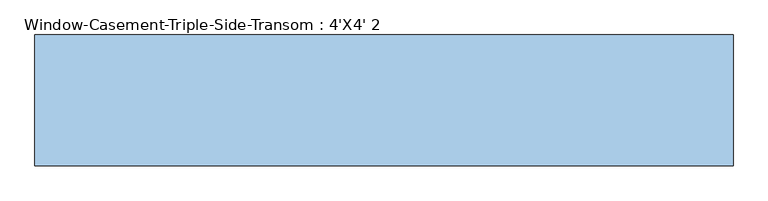
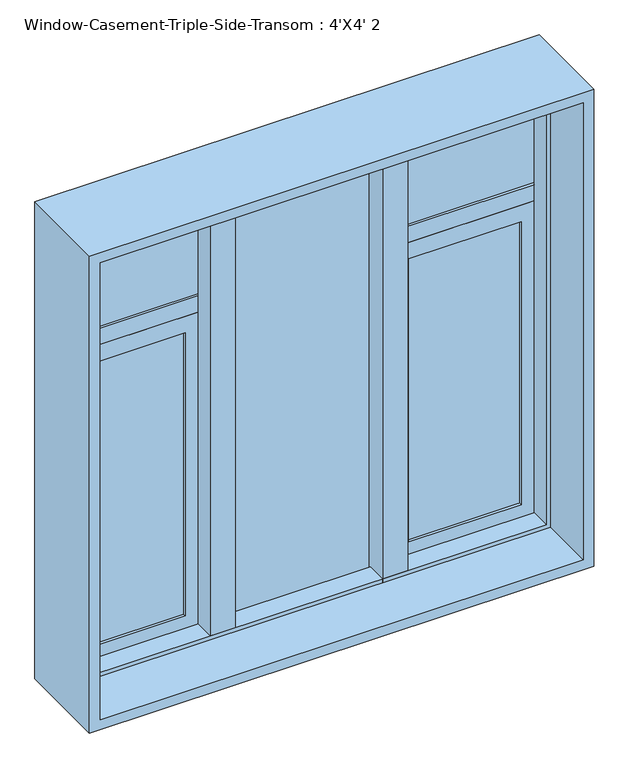
"""IFC4 building model written with IfcOpenShell, lengths in millimetres: window geometry, Window-Casement-Triple-Side-Transom : 4'X4' 2."""

from ifc_helpers import new_model, si_unit, frame, origin, place, context, project, spatial, polyline, outline, extrude, faceted_brep, source, transform, mapped, element, save


def window_casement_triple_side_transom_4_x4_2_fd24aed3(model_context):
    return source(origin(), model_context, "Body", "SolidModel", [
        faceted_brep([(-584.2, 73.025, 2108.2), (-584.2, 114.3, 2108.2), (584.2, 114.3, 2108.2), (584.2, 73.025, 2108.2), (-574.0796875, 22.225, 2098.0796875), (-574.0796875, 73.025, 2098.0796875), (574.0796875, 73.025, 2098.0796875), (574.0796875, 22.225, 2098.0796875), (-584.2, -114.3, 2108.2), (-584.2, 22.225, 2108.2), (584.2, 22.225, 2108.2), (584.2, -114.3, 2108.2), (-609.6, 114.3, 2133.6), (-609.6, -114.3, 2133.6), (609.6, -114.3, 2133.6), (609.6, 114.3, 2133.6), (584.2, 114.3, 939.8), (584.2, 73.025, 939.8), (574.0796875, 73.025, 949.9203125), (574.0796875, 22.225, 949.9203125), (584.2, 22.225, 939.8), (584.2, -114.3, 939.8), (609.6, -114.3, 914.4), (609.6, 114.3, 914.4), (-584.2, 114.3, 939.8), (-584.2, 73.025, 939.8), (-574.0796875, 73.025, 949.9203125), (-574.0796875, 22.225, 949.9203125), (-584.2, 22.225, 939.8), (-584.2, -114.3, 939.8), (-609.6, -114.3, 914.4), (-609.6, 114.3, 914.4)], [[[0, 1, 2, 3]], [[4, 5, 6, 7]], [[8, 9, 10, 11]], [[12, 13, 14, 15]], [[3, 2, 16, 17]], [[7, 6, 18, 19]], [[11, 10, 20, 21]], [[15, 14, 22, 23]], [[17, 16, 24, 25]], [[19, 18, 26, 27]], [[21, 20, 28, 29]], [[23, 22, 30, 31]], [[25, 24, 1, 0]], [[3, 17, 25, 0], [5, 26, 18, 6]], [[27, 26, 5, 4]], [[9, 28, 20, 10], [7, 19, 27, 4]], [[29, 28, 9, 8]], [[13, 30, 22, 14], [11, 21, 29, 8]], [[31, 30, 13, 12]], [[15, 23, 31, 12], [1, 24, 16, 2]]]),
        extrude(outline(polyline([(-177.8, 111.125), (-177.8, 22.225), (-238.7203125, 22.225), (-238.7203125, 73.025), (-228.6, 73.025), (-228.6, 111.125), (-177.8, 111.125)])), frame((0.0, 0.0, 939.8), z_axis=(0.0, 0.0, 1.0), x_axis=(1.0, 0.0, 0.0)), (0.0, 0.0, 1.0), 1168.4),
        extrude(outline(polyline([(228.6, 111.125), (228.6, 73.025), (238.7203125, 73.025), (238.7203125, 22.225), (177.8, 22.225), (177.8, 111.125), (228.6, 111.125)])), frame((0.0, 0.0, 939.8), z_axis=(0.0, 0.0, 1.0), x_axis=(1.0, 0.0, 0.0)), (0.0, 0.0, 1.0), 1168.4),
        extrude(outline(polyline([(1746.9048438, 228.6), (939.8, 228.6), (939.8, 584.2), (1746.9048438, 584.2), (1746.9048438, 228.6)]), holes=[polyline([(1705.0345313, 542.3296875), (981.6703125, 542.3296875), (981.6703125, 270.4703125), (1705.0345313, 270.4703125), (1705.0345313, 542.3296875)])]), frame((0.0, 73.025, 0.0), z_axis=(0.0, 1.0, 0.0), x_axis=(0.0, 0.0, 1.0)), (0.0, 0.0, 1.0), 31.75),
        extrude(outline(polyline([(1746.9048438, -584.2), (939.8, -584.2), (939.8, -228.6), (1746.9048438, -228.6), (1746.9048438, -584.2)]), holes=[polyline([(1705.0345313, -270.4703125), (981.6703125, -270.4703125), (981.6703125, -542.3296875), (1705.0345313, -542.3296875), (1705.0345313, -270.4703125)])]), frame((0.0, 73.025, 0.0), z_axis=(0.0, 1.0, 0.0), x_axis=(0.0, 0.0, 1.0)), (0.0, 0.0, 1.0), 31.75),
        extrude(outline(polyline([(-270.4703125, 98.425), (-270.4703125, 92.075), (-542.3296875, 92.075), (-542.3296875, 98.425), (-270.4703125, 98.425)])), frame((0.0, 0.0, 981.6703125), z_axis=(0.0, 0.0, 1.0), x_axis=(1.0, 0.0, 0.0)), (0.0, 0.0, 1.0), 723.3642188),
        extrude(outline(polyline([(-270.4703125, 85.725), (-270.4703125, 79.375), (-542.3296875, 79.375), (-542.3296875, 85.725), (-270.4703125, 85.725)])), frame((0.0, 0.0, 981.6703125), z_axis=(0.0, 0.0, 1.0), x_axis=(1.0, 0.0, 0.0)), (0.0, 0.0, 1.0), 723.3642188),
        extrude(outline(polyline([(542.3296875, 98.425), (542.3296875, 92.075), (270.4703125, 92.075), (270.4703125, 98.425), (542.3296875, 98.425)])), frame((0.0, 0.0, 981.6703125), z_axis=(0.0, 0.0, 1.0), x_axis=(1.0, 0.0, 0.0)), (0.0, 0.0, 1.0), 723.3642188),
        extrude(outline(polyline([(542.3296875, 85.725), (542.3296875, 79.375), (270.4703125, 79.375), (270.4703125, 85.725), (542.3296875, 85.725)])), frame((0.0, 0.0, 981.6703125), z_axis=(0.0, 0.0, 1.0), x_axis=(1.0, 0.0, 0.0)), (0.0, 0.0, 1.0), 723.3642188),
        extrude(outline(polyline([(584.2, 104.775), (584.2, 73.025), (228.6, 73.025), (228.6, 104.775), (584.2, 104.775)])), frame((0.0, 0.0, 1746.9048438), z_axis=(0.0, 0.0, 1.0), x_axis=(1.0, 0.0, 0.0)), (0.0, 0.0, 1.0), 41.8703125),
        extrude(outline(polyline([(177.8, 98.425), (177.8, 92.075), (-177.8, 92.075), (-177.8, 98.425), (177.8, 98.425)])), frame((0.0, 0.0, 939.8), z_axis=(0.0, 0.0, 1.0), x_axis=(1.0, 0.0, 0.0)), (0.0, 0.0, 1.0), 1168.4),
        extrude(outline(polyline([(177.8, 85.725), (177.8, 79.375), (-177.8, 79.375), (-177.8, 85.725), (177.8, 85.725)])), frame((0.0, 0.0, 939.8), z_axis=(0.0, 0.0, 1.0), x_axis=(1.0, 0.0, 0.0)), (0.0, 0.0, 1.0), 1168.4),
        extrude(outline(polyline([(-228.6, 104.775), (-228.6, 73.025), (-584.2, 73.025), (-584.2, 104.775), (-228.6, 104.775)])), frame((0.0, 0.0, 1746.9048438), z_axis=(0.0, 0.0, 1.0), x_axis=(1.0, 0.0, 0.0)), (0.0, 0.0, 1.0), 41.8703125),
        extrude(outline(polyline([(-228.6, 98.425), (-228.6, 92.075), (-584.2, 92.075), (-584.2, 98.425), (-228.6, 98.425)])), frame((0.0, 0.0, 1788.7751562), z_axis=(0.0, 0.0, 1.0), x_axis=(1.0, 0.0, 0.0)), (0.0, 0.0, 1.0), 319.4248438),
        extrude(outline(polyline([(-228.6, 85.725), (-228.6, 79.375), (-584.2, 79.375), (-584.2, 85.725), (-228.6, 85.725)])), frame((0.0, 0.0, 1788.7751562), z_axis=(0.0, 0.0, 1.0), x_axis=(1.0, 0.0, 0.0)), (0.0, 0.0, 1.0), 319.4248438),
        extrude(outline(polyline([(584.2, 98.425), (584.2, 92.075), (228.6, 92.075), (228.6, 98.425), (584.2, 98.425)])), frame((0.0, 0.0, 1788.7751562), z_axis=(0.0, 0.0, 1.0), x_axis=(1.0, 0.0, 0.0)), (0.0, 0.0, 1.0), 319.4248438),
        extrude(outline(polyline([(584.2, 85.725), (584.2, 79.375), (228.6, 79.375), (228.6, 85.725), (584.2, 85.725)])), frame((0.0, 0.0, 1788.7751562), z_axis=(0.0, 0.0, 1.0), x_axis=(1.0, 0.0, 0.0)), (0.0, 0.0, 1.0), 319.4248438),
    ])


if __name__ == "__main__":
    model = new_model("IFC4")
    model_context = context("Model", 3, world=origin())
    ifc_project = project(units=[si_unit("LENGTHUNIT", "METRE", prefix="MILLI")], contexts=[model_context])
    site = spatial("IfcSite", under=ifc_project)
    building = spatial("IfcBuilding", under=site)
    placement = place(None, origin())
    window_casement_triple_side_transom_4_x4_2_shape = window_casement_triple_side_transom_4_x4_2_fd24aed3(model_context)
    element("IfcWindow", 1, ObjectType="Window-Casement-Triple-Side-Transom : 4'X4' 2", at=placement, inside=building, context=model_context, shape_type="MappedRepresentation", body=[
        mapped(window_casement_triple_side_transom_4_x4_2_shape, transform((0.0, 0.0, 0.0), x_axis=(1.0, 0.0, 0.0), y_axis=(0.0, 1.0, 0.0), z_axis=(0.0, 0.0, 1.0))),
    ])
    save(model, "model.ifc")

# Revit data of these elements
# Type "Window-Casement-Triple-Side-Transom : 4'X4' 2"
#   Type Mark = "26"
#   Fire Rating = "0.5h"
#   Assembly Code = "B2020100"
#   Analytic Construction = "Double glazing - domestic"
#   Window Width = 1' - 4"
#   Window Inset [instance default] = 0' - 0 5/8"
#   Wall Thickness [instance default] = 0' - 6"
#   Visual Light Transmittance = 0.81
#   Transom Height Ratio = 0.3
#   Thermal Resistance (R) = 1.8146 (h·ft²·°F)/BTU
#   Solar Heat Gain Coefficient = 0.76
#   Rough Width = 4' - 0 1/2"
#   Rough Height = 4' - 0 1/2"
#   Open Window Height = 2' - 9.6"
#   Heat Transfer Coefficient (U) = 0.5511 BTU/(h·ft²·°F)
#   Height = 4' - 0"
#   Transom Height = 1' - 2.4"
#   Frame Gap 3 [instance default] = 0' - 1 83/128"
#   Frame Gap 2 [instance default] = 0' - 0 5/8"
#   Frame Gap 1 = 0' - 1 51/128"
#   Default Sill Height = 3' - 0"
#   Width = 4' - 0"
#   Frame Material = Metal - Aluminum
#   Glass Panel Material = Glass
#   Wall Closure = (empty or 0)
# Element 1 (IfcWindow, "Window-Casement-Triple-Side-Transom : 4'X4' 2")
#   Wall Thickness = 0' - 9"
#   Materials on its faces: "Metal - Aluminum", "Glass"
# Materials
#   "Metal - Aluminum": class "Metal", colour RGB 247 247 247, transparency 0
#   "Glass": class "Glass", colour RGB 0 128 192, transparency 0.75, Description = "Soda Lime Glass", Cost = 0
